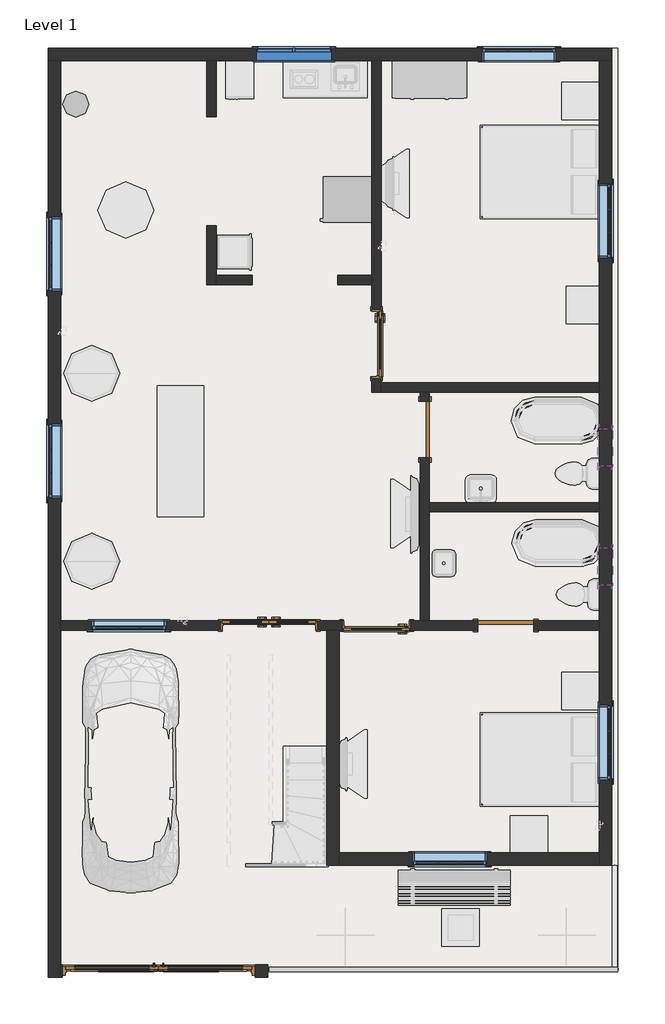
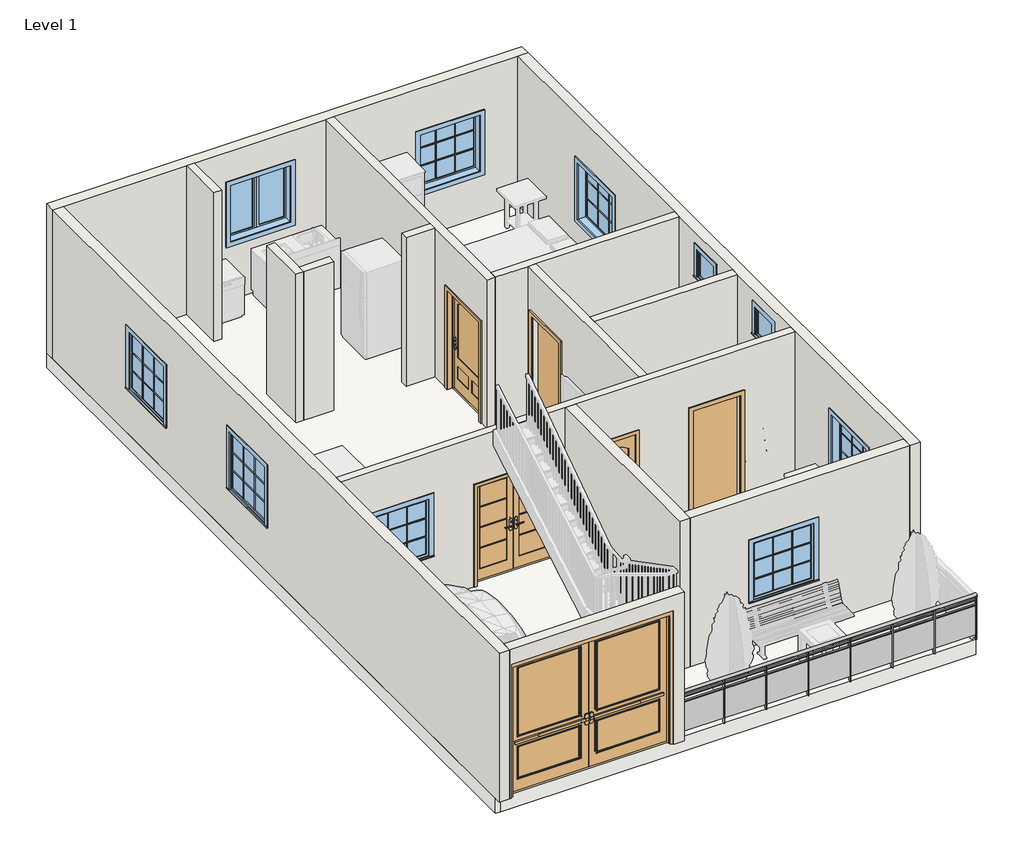
# One storey, part 1 of 3: 15 walls, 10 windows, 6 doors, 1 railing, 1 slab.
"""IFC4 building model written with IfcOpenShell, lengths in millimetres."""

from ifc_helpers import new_model, si_unit, point, frame, origin, origin_with_axes, place, context, project, spatial, polyline, ellipse_curve, trimmed, outline, extrude, faceted_brep, transform, mapped, element, save
from ifc_brep_helpers import plane_surface, extruded_surface, advanced_brep
from components import door_25c67de5, door_94998e6c, door_7b75190e, door_e43601eb, door_2971dfc0, door_686f89d2, window_7418cbd4, window_7e6ae3b0, window_0862ab64, window_e41d21a6

model = new_model("IFC4")

# Units and contexts
model_context = context("Model", 3, world=origin())
ifc_project = project(units=[si_unit("LENGTHUNIT", "METRE", prefix="MILLI")], contexts=[model_context])

# Site, building, storey
site = spatial("IfcSite", under=ifc_project)
building = spatial("IfcBuilding", under=site)
storey = spatial("IfcBuildingStorey", under=building, Name="Level 1", Elevation=0.0)

# Doors
placement = place(None, origin())
door_shape = door_25c67de5(model_context)
element("IfcDoor", 1, ObjectType="42\" x 80\"", at=placement, inside=storey, context=model_context, shape_type="MappedRepresentation", body=[
    mapped(door_shape, transform((-10170.509927, 3983.7437882, 0.0), x_axis=(1.0, 0.0, 0.0), y_axis=(0.0, 1.0, 0.0), z_axis=(0.0, 0.0, 1.0))),
])
element("IfcDoor", 2, ObjectType="42\" x 80\"", at=placement, inside=storey, context=model_context, shape_type="MappedRepresentation", body=[
    mapped(door_shape, transform((-10167.334927, 8584.3187882, 0.0), x_axis=(0.0, 1.0, 0.0), y_axis=(-1.0, 0.0, 0.0), z_axis=(0.0, 0.0, 1.0))),
])
door_2_shape = door_94998e6c(model_context)
element("IfcDoor", 3, ObjectType="Door-Exterior-Double-Full Glass-Wood_Clad : 60\" x 80\"", at=placement, inside=storey, context=model_context, shape_type="MappedRepresentation", body=[
    mapped(door_2_shape, transform((-11923.109927, 3990.0937882, 0.0), x_axis=(1.0, 0.0, 0.0), y_axis=(0.0, 1.0, 0.0), z_axis=(0.0, 0.0, 1.0))),
])
door_3_shape = door_7b75190e(model_context)
door_4_shape = door_e43601eb(model_context)
door_5_shape = door_2971dfc0(model_context)
element("IfcDoor", 4, ObjectType="Door-Exterior-Double-Two_Lite : 120\" x 104\"", at=placement, inside=storey, context=model_context, shape_type="MappedRepresentation", body=[
    mapped(door_3_shape, transform((-13726.509927, -1658.2312118, 0.0), x_axis=(1.0, 0.0, 0.0), y_axis=(0.0, 1.0, 0.0), z_axis=(0.0, 0.0, 1.0))),
    mapped(door_4_shape, transform((-13726.509927, -1658.2312118, 0.0), x_axis=(1.0, 0.0, 0.0), y_axis=(0.0, 1.0, 0.0), z_axis=(0.0, 0.0, 1.0))),
    mapped(door_5_shape, transform((-13726.509927, -1658.2312118, 0.0), x_axis=(1.0, 0.0, 0.0), y_axis=(0.0, 1.0, 0.0), z_axis=(0.0, 0.0, 1.0))),
])
door_6_shape = door_686f89d2(model_context)
element("IfcDoor", 5, ObjectType="Single-Flush : 36\" x 84\"", at=placement, inside=storey, context=model_context, shape_type="MappedRepresentation", body=[
    mapped(door_6_shape, transform((-9383.109927, 7187.3187882, 0.0), x_axis=(0.0, 1.0, 0.0), y_axis=(-1.0, 0.0, 0.0), z_axis=(0.0, 0.0, 1.0))),
])
element("IfcDoor", 6, ObjectType="Single-Flush : 36\" x 84\"", at=placement, inside=storey, context=model_context, shape_type="MappedRepresentation", body=[
    mapped(door_6_shape, transform((-8062.309927, 3986.9187882, 0.0), x_axis=(-1.0, 0.0, 0.0), y_axis=(0.0, -1.0, 0.0), z_axis=(0.0, 0.0, 1.0))),
])

# Railing
element("IfcRailing", 7, ObjectType="Glass Panel - Bottom Fill", at=placement, inside=storey, context=model_context, shape_type="SolidModel", body=[
    advanced_brep(
    [(-6233.509927, -1659.8187118, 914.4), (-6233.509927, -1583.6187118, 914.4), (-11923.109927, -1659.8187118, 914.4), (-11923.109927, -1583.6187118, 914.4)],
    [
        (0, 1, ellipse_curve(frame((-6233.509927, -1621.7187118, 914.4), z_axis=(1.0, 0.0, 0.0), x_axis=(0.0, 1.0, 0.0)), 38.1, 28.575)),
        (1, 0, ellipse_curve(frame((-6233.509927, -1621.7187118, 914.4), z_axis=(1.0, 0.0, 0.0), x_axis=(0.0, 1.0, 0.0)), 38.1, 28.575)),
        (2, 3, ellipse_curve(frame((-11923.109927, -1621.7187118, 914.4), z_axis=(-1.0, 0.0, 0.0), x_axis=(0.0, 1.0, 0.0)), 38.1, 28.575)),
        (3, 2, ellipse_curve(frame((-11923.109927, -1621.7187118, 914.4), z_axis=(-1.0, 0.0, 0.0), x_axis=(0.0, 1.0, 0.0)), 38.1, 28.575)),
        (0, 2),
        (3, 1),
    ],
    [
        plane_surface(frame((-6233.509927, -1621.7187118, 914.4), z_axis=(1.0, 0.0, 0.0), x_axis=(0.0, -1.0, 0.0))),
        plane_surface(frame((-11923.109927, -1621.7187118, 914.4), z_axis=(-1.0, 0.0, 0.0), x_axis=(0.0, -1.0, 0.0))),
        extruded_surface(trimmed(ellipse_curve(frame((-11923.109927, -1621.7187118, 914.4), z_axis=(1.0, 0.0, 0.0), x_axis=(0.0, 1.0, 0.0)), 38.1, 28.575), [point((-11923.109927, -1659.8187118, 914.4))], [point((-11923.109927, -1583.6187118, 914.4))], True, "CARTESIAN"), (5689.599999999999, 0.0, 0.0), 5689.599999999999),
        extruded_surface(trimmed(ellipse_curve(frame((-11923.109927, -1621.7187118, 914.4), z_axis=(1.0, 0.0, 0.0), x_axis=(0.0, 1.0, 0.0)), 38.1, 28.575), [point((-11923.109927, -1583.6187118, 914.4))], [point((-11923.109927, -1659.8187118, 914.4))], True, "CARTESIAN"), (5689.599999999999, 0.0, 0.0), 5689.599999999999),
    ],
    [
        (0, [[1, 2]]),
        (1, [[3, 4]]),
        (2, [[-1, 5, -4, 6]]),
        (3, [[-2, -6, -3, -5]]),
    ],
),
    extrude(outline(polyline([(-6233.509927, -1609.0187118), (-6233.509927, -1634.4187118), (-11923.109927, -1634.4187118), (-11923.109927, -1609.0187118), (-6233.509927, -1609.0187118)])), frame((0.0, 0.0, 800.1), z_axis=(0.0, 0.0, 1.0), x_axis=(1.0, 0.0, 0.0)), (0.0, 0.0, 1.0), 25.4),
    extrude(outline(polyline([(-6233.509927, -1609.0187118), (-6233.509927, -1634.4187118), (-11923.109927, -1634.4187118), (-11923.109927, -1609.0187118), (-6233.509927, -1609.0187118)])), frame((0.0, 0.0, 698.5), z_axis=(0.0, 0.0, 1.0), x_axis=(1.0, 0.0, 0.0)), (0.0, 0.0, 1.0), 25.4),
    extrude(outline(polyline([(-11110.309927, -1628.2538688), (-11923.109927, -1628.2538688), (-11923.109927, -1621.9038688), (-11110.309927, -1621.9038688), (-11110.309927, -1628.2538688)])), frame((0.0, 0.0, 101.6), z_axis=(0.0, 0.0, 1.0), x_axis=(1.0, 0.0, 0.0)), (0.0, 0.0, 1.0), 596.9),
    extrude(outline(polyline([(-11103.959927, -1596.3187118), (-11103.959927, -1647.1187118), (-11116.659927, -1647.1187118), (-11116.659927, -1596.3187118), (-11103.959927, -1596.3187118)])), origin_with_axes(), (0.0, 0.0, 1.0), 885.6788223),
    extrude(outline(polyline([(-10297.509927, -1628.2538688), (-11110.309927, -1628.2538688), (-11110.309927, -1621.9038688), (-10297.509927, -1621.9038688), (-10297.509927, -1628.2538688)])), frame((0.0, 0.0, 101.6), z_axis=(0.0, 0.0, 1.0), x_axis=(1.0, 0.0, 0.0)), (0.0, 0.0, 1.0), 596.9),
    extrude(outline(polyline([(-10291.159927, -1596.3187118), (-10291.159927, -1647.1187118), (-10303.859927, -1647.1187118), (-10303.859927, -1596.3187118), (-10291.159927, -1596.3187118)])), origin_with_axes(), (0.0, 0.0, 1.0), 885.6788223),
    extrude(outline(polyline([(-9484.709927, -1628.2538688), (-10297.509927, -1628.2538688), (-10297.509927, -1621.9038688), (-9484.709927, -1621.9038688), (-9484.709927, -1628.2538688)])), frame((0.0, 0.0, 101.6), z_axis=(0.0, 0.0, 1.0), x_axis=(1.0, 0.0, 0.0)), (0.0, 0.0, 1.0), 596.9),
    extrude(outline(polyline([(-9478.359927, -1596.3187118), (-9478.359927, -1647.1187118), (-9491.059927, -1647.1187118), (-9491.059927, -1596.3187118), (-9478.359927, -1596.3187118)])), origin_with_axes(), (0.0, 0.0, 1.0), 885.6788223),
    extrude(outline(polyline([(-8671.909927, -1628.2538688), (-9484.709927, -1628.2538688), (-9484.709927, -1621.9038688), (-8671.909927, -1621.9038688), (-8671.909927, -1628.2538688)])), frame((0.0, 0.0, 101.6), z_axis=(0.0, 0.0, 1.0), x_axis=(1.0, 0.0, 0.0)), (0.0, 0.0, 1.0), 596.9),
    extrude(outline(polyline([(-8665.559927, -1596.3187118), (-8665.559927, -1647.1187118), (-8678.259927, -1647.1187118), (-8678.259927, -1596.3187118), (-8665.559927, -1596.3187118)])), origin_with_axes(), (0.0, 0.0, 1.0), 885.6788223),
    extrude(outline(polyline([(-7859.109927, -1628.2538688), (-8671.909927, -1628.2538688), (-8671.909927, -1621.9038688), (-7859.109927, -1621.9038688), (-7859.109927, -1628.2538688)])), frame((0.0, 0.0, 101.6), z_axis=(0.0, 0.0, 1.0), x_axis=(1.0, 0.0, 0.0)), (0.0, 0.0, 1.0), 596.9),
    extrude(outline(polyline([(-7852.759927, -1596.3187118), (-7852.759927, -1647.1187118), (-7865.459927, -1647.1187118), (-7865.459927, -1596.3187118), (-7852.759927, -1596.3187118)])), origin_with_axes(), (0.0, 0.0, 1.0), 885.6788223),
    extrude(outline(polyline([(-7046.309927, -1628.2538688), (-7859.109927, -1628.2538688), (-7859.109927, -1621.9038688), (-7046.309927, -1621.9038688), (-7046.309927, -1628.2538688)])), frame((0.0, 0.0, 101.6), z_axis=(0.0, 0.0, 1.0), x_axis=(1.0, 0.0, 0.0)), (0.0, 0.0, 1.0), 596.9),
    extrude(outline(polyline([(-7039.959927, -1596.3187118), (-7039.959927, -1647.1187118), (-7052.659927, -1647.1187118), (-7052.659927, -1596.3187118), (-7039.959927, -1596.3187118)])), origin_with_axes(), (0.0, 0.0, 1.0), 885.6788223),
    extrude(outline(polyline([(-6233.509927, -1628.2538688), (-7046.309927, -1628.2538688), (-7046.309927, -1621.9038688), (-6233.509927, -1621.9038688), (-6233.509927, -1628.2538688)])), frame((0.0, 0.0, 101.6), z_axis=(0.0, 0.0, 1.0), x_axis=(1.0, 0.0, 0.0)), (0.0, 0.0, 1.0), 596.9),
    extrude(outline(polyline([(-11910.409927, -1612.1937118), (-11910.409927, -1631.2437118), (-11929.459927, -1631.2437118), (-11929.459927, -1612.1937118), (-11910.409927, -1612.1937118)])), origin_with_axes(), (0.0, 0.0, 1.0), 885.6788223),
    extrude(outline(polyline([(-6227.159927, -1612.1937118), (-6227.159927, -1631.2437118), (-6246.209927, -1631.2437118), (-6246.209927, -1612.1937118), (-6227.159927, -1612.1937118)])), origin_with_axes(), (0.0, 0.0, 1.0), 885.6788223),
])

# Slab
element("IfcSlab", 8, ObjectType="Generic - 12\"", at=placement, inside=storey, context=model_context, shape_type="SweptSolid", body=[
    extrude(outline(polyline([(-6233.509927, 13410.3187882), (-6233.509927, -1621.7187118), (-15428.309927, -1621.7187118), (-15529.909927, -1621.7187118), (-15529.909927, 13410.3187882), (-6233.509927, 13410.3187882)])), frame((0.0, 0.0, -304.8), z_axis=(0.0, 0.0, 1.0), x_axis=(1.0, 0.0, 0.0)), (0.0, 0.0, 1.0), 304.8),
])

# Walls
element("IfcWall", 9, ObjectType="Generic - 8\"", at=placement, inside=storey, context=model_context, shape_type="Brep", body=[
    faceted_brep([(-15529.909927, 13207.1187882, 0.0), (-15326.709927, 13207.1187882, 0.0), (-12939.109927, 13207.1187882, 0.0), (-12786.709927, 13207.1187882, 0.0), (-10246.709927, 13207.1187882, 0.0), (-10094.309927, 13207.1187882, 0.0), (-6538.309927, 13207.1187882, 0.0), (-6335.109927, 13207.1187882, 0.0), (-6335.109927, 13207.1187882, 3048.0), (-6538.309927, 13207.1187882, 3048.0), (-10094.309927, 13207.1187882, 3048.0), (-10246.709927, 13207.1187882, 3048.0), (-12786.709927, 13207.1187882, 3048.0), (-12939.109927, 13207.1187882, 3048.0), (-15326.709927, 13207.1187882, 3048.0), (-15529.909927, 13207.1187882, 3048.0), (-7236.809927, 13207.1187882, 2133.6), (-7236.809927, 13207.1187882, 914.4), (-8456.009927, 13207.1187882, 914.4), (-8456.009927, 13207.1187882, 2133.6), (-10907.109927, 13207.1187882, 2387.6), (-10907.109927, 13207.1187882, 1168.4), (-12126.309927, 13207.1187882, 1168.4), (-12126.309927, 13207.1187882, 2387.6), (-15529.909927, 13410.3187882, 0.0), (-15529.909927, 13410.3187882, 3048.0), (-6335.109927, 13410.3187882, 3048.0), (-6335.109927, 13410.3187882, 0.0), (-7236.809927, 13410.3187882, 2133.6), (-8456.009927, 13410.3187882, 2133.6), (-8456.009927, 13410.3187882, 914.4), (-7236.809927, 13410.3187882, 914.4), (-10907.109927, 13410.3187882, 2387.6), (-12126.309927, 13410.3187882, 2387.6), (-12126.309927, 13410.3187882, 1168.4), (-10907.109927, 13410.3187882, 1168.4)], [[[0, 1, 2, 3, 4, 5, 6, 7, 8, 9, 10, 11, 12, 13, 14, 15], [16, 17, 18, 19], [20, 21, 22, 23]], [[24, 25, 26, 27], [28, 29, 30, 31], [32, 33, 34, 35]], [[7, 6, 5, 4, 3, 2, 1, 0, 24, 27]], [[15, 14, 13, 12, 11, 10, 9, 8, 26, 25]], [[8, 7, 27, 26]], [[0, 15, 25, 24]], [[17, 16, 28, 31]], [[18, 17, 31, 30]], [[19, 18, 30, 29]], [[16, 19, 29, 28]], [[21, 20, 32, 35]], [[22, 21, 35, 34]], [[23, 22, 34, 33]], [[20, 23, 33, 32]]]),
])
element("IfcWall", 10, ObjectType="Generic - 8\"", at=placement, inside=storey, context=model_context, shape_type="Brep", body=[
    faceted_brep([(-6538.309927, 13207.1187882, 0.0), (-6538.309927, 7949.3187882, 0.0), (-6538.309927, 7796.9187882, 0.0), (-6538.309927, 5993.5187882, 0.0), (-6538.309927, 5841.1187882, 0.0), (-6538.309927, 4063.1187882, 0.0), (-6538.309927, 3910.7187882, 0.0), (-6538.309927, 278.5187882, 0.0), (-6538.309927, 75.3187882, 0.0), (-6538.309927, 75.3187882, 3048.0), (-6538.309927, 278.5187882, 3048.0), (-6538.309927, 3910.7187882, 3048.0), (-6538.309927, 4063.1187882, 3048.0), (-6538.309927, 5841.1187882, 3048.0), (-6538.309927, 5993.5187882, 3048.0), (-6538.309927, 7796.9187882, 3048.0), (-6538.309927, 7949.3187882, 3048.0), (-6538.309927, 13207.1187882, 3048.0), (-6538.309927, 1472.3187882, 2133.6), (-6538.309927, 1472.3187882, 914.4), (-6538.309927, 2691.5187882, 914.4), (-6538.309927, 2691.5187882, 2133.6), (-6538.309927, 9981.3187882, 2133.6), (-6538.309927, 9981.3187882, 914.4), (-6538.309927, 11200.5187882, 914.4), (-6538.309927, 11200.5187882, 2133.6), (-6538.309927, 7200.0187882, 2768.6), (-6538.309927, 6590.4187882, 2768.6), (-6538.309927, 6590.4187882, 2159.0), (-6538.309927, 7200.0187882, 2159.0), (-6538.309927, 5256.9187882, 2768.6), (-6538.309927, 4647.3187882, 2768.6), (-6538.309927, 4647.3187882, 2159.0), (-6538.309927, 5256.9187882, 2159.0), (-6335.109927, 13207.1187882, 0.0), (-6335.109927, 13207.1187882, 3048.0), (-6335.109927, 75.3187882, 3048.0), (-6335.109927, 75.3187882, 0.0), (-6335.109927, 1472.3187882, 2133.6), (-6335.109927, 2691.5187882, 2133.6), (-6335.109927, 2691.5187882, 914.4), (-6335.109927, 1472.3187882, 914.4), (-6335.109927, 9981.3187882, 2133.6), (-6335.109927, 11200.5187882, 2133.6), (-6335.109927, 11200.5187882, 914.4), (-6335.109927, 9981.3187882, 914.4), (-6335.109927, 7200.0187882, 2768.6), (-6335.109927, 7200.0187882, 2159.0), (-6335.109927, 6590.4187882, 2159.0), (-6335.109927, 6590.4187882, 2768.6), (-6335.109927, 5256.9187882, 2768.6), (-6335.109927, 5256.9187882, 2159.0), (-6335.109927, 4647.3187882, 2159.0), (-6335.109927, 4647.3187882, 2768.6)], [[[0, 1, 2, 3, 4, 5, 6, 7, 8, 9, 10, 11, 12, 13, 14, 15, 16, 17], [18, 19, 20, 21], [22, 23, 24, 25], [26, 27, 28, 29], [30, 31, 32, 33]], [[34, 35, 36, 37], [38, 39, 40, 41], [42, 43, 44, 45], [46, 47, 48, 49], [50, 51, 52, 53]], [[8, 7, 6, 5, 4, 3, 2, 1, 0, 34, 37]], [[17, 16, 15, 14, 13, 12, 11, 10, 9, 36, 35]], [[0, 17, 35, 34]], [[9, 8, 37, 36]], [[19, 18, 38, 41]], [[20, 19, 41, 40]], [[21, 20, 40, 39]], [[18, 21, 39, 38]], [[23, 22, 42, 45]], [[24, 23, 45, 44]], [[25, 24, 44, 43]], [[22, 25, 43, 42]], [[47, 46, 26, 29]], [[48, 47, 29, 28]], [[49, 48, 28, 27]], [[46, 49, 27, 26]], [[51, 50, 30, 33]], [[52, 51, 33, 32]], [[53, 52, 32, 31]], [[50, 53, 31, 30]]]),
])
element("IfcWall", 11, ObjectType="Generic - 8\"", at=placement, inside=storey, context=model_context, shape_type="SweptSolid", body=[
    extrude(outline(polyline([(0.0, -6538.309927), (3048.0, -6538.309927), (3048.0, -10780.109927), (0.0, -10780.109927), (0.0, -6538.309927)]), holes=[polyline([(2133.6, -9586.309927), (2133.6, -8367.109927), (914.4, -8367.109927), (914.4, -9586.309927), (2133.6, -9586.309927)])]), frame((0.0, 75.3187882, 0.0), z_axis=(0.0, 1.0, 0.0), x_axis=(0.0, 0.0, 1.0)), (0.0, 0.0, 1.0), 203.2),
])
element("IfcWall", 12, ObjectType="Generic - 8\"", at=placement, inside=storey, context=model_context, shape_type="Brep", body=[
    faceted_brep([(-15326.709927, -1753.4812118, 0.0), (-15326.709927, -1550.2812118, 0.0), (-15326.709927, 3910.7187882, 0.0), (-15326.709927, 4063.1187882, 0.0), (-15326.709927, 13207.1187882, 0.0), (-15326.709927, 13207.1187882, 3048.0), (-15326.709927, 4063.1187882, 3048.0), (-15326.709927, 3910.7187882, 3048.0), (-15326.709927, -1550.2812118, 3048.0), (-15326.709927, -1753.4812118, 3048.0), (-15326.709927, 7282.5687882, 2133.6), (-15326.709927, 7282.5687882, 914.4), (-15326.709927, 6063.3687882, 914.4), (-15326.709927, 6063.3687882, 2133.6), (-15326.709927, 10660.7687882, 2133.6), (-15326.709927, 10660.7687882, 914.4), (-15326.709927, 9441.5687882, 914.4), (-15326.709927, 9441.5687882, 2133.6), (-15529.909927, -1753.4812118, 0.0), (-15529.909927, -1753.4812118, 3048.0), (-15529.909927, 13207.1187882, 3048.0), (-15529.909927, 13207.1187882, 0.0), (-15529.909927, 7282.5687882, 2133.6), (-15529.909927, 6063.3687882, 2133.6), (-15529.909927, 6063.3687882, 914.4), (-15529.909927, 7282.5687882, 914.4), (-15529.909927, 10660.7687882, 2133.6), (-15529.909927, 9441.5687882, 2133.6), (-15529.909927, 9441.5687882, 914.4), (-15529.909927, 10660.7687882, 914.4)], [[[0, 1, 2, 3, 4, 5, 6, 7, 8, 9], [10, 11, 12, 13], [14, 15, 16, 17]], [[18, 19, 20, 21], [22, 23, 24, 25], [26, 27, 28, 29]], [[4, 3, 2, 1, 0, 18, 21]], [[9, 8, 7, 6, 5, 20, 19]], [[5, 4, 21, 20]], [[11, 10, 22, 25]], [[12, 11, 25, 24]], [[13, 12, 24, 23]], [[10, 13, 23, 22]], [[15, 14, 26, 29]], [[16, 15, 29, 28]], [[17, 16, 28, 27]], [[14, 17, 27, 26]], [[0, 9, 19, 18]]]),
])
element("IfcWall", 13, ObjectType="Generic - 8\"", at=placement, inside=storey, context=model_context, shape_type="Brep", body=[
    faceted_brep([(-10983.309927, 3910.7187882, 0.0), (-10983.309927, 75.3187882, 0.0), (-10983.309927, 75.3187882, 3048.0), (-10983.309927, 3910.7187882, 3048.0), (-10780.109927, 3910.7187882, 0.0), (-10780.109927, 3910.7187882, 3048.0), (-10780.109927, 278.5187882, 3048.0), (-10780.109927, 75.3187882, 3048.0), (-10780.109927, 75.3187882, 0.0), (-10780.109927, 278.5187882, 0.0)], [[[0, 1, 2, 3]], [[4, 5, 6, 7, 8, 9]], [[1, 0, 4, 9, 8]], [[3, 2, 7, 6, 5]], [[0, 3, 5, 4]], [[2, 1, 8, 7]]]),
])
element("IfcWall", 14, ObjectType="Generic - 8\"", at=placement, inside=storey, context=model_context, shape_type="SweptSolid", body=[
    extrude(outline(polyline([(0.0, -11948.509927), (3048.0, -11948.509927), (3048.0, -15326.709927), (0.0, -15326.709927), (0.0, -15301.309927), (2743.2, -15301.309927), (2743.2, -12151.709927), (0.0, -12151.709927), (0.0, -11948.509927)])), frame((0.0, -1753.4812118, 0.0), z_axis=(0.0, 1.0, 0.0), x_axis=(0.0, 0.0, 1.0)), (0.0, 0.0, 1.0), 203.2),
])
element("IfcWall", 15, ObjectType="INNER WALL", at=placement, inside=storey, context=model_context, shape_type="Brep", body=[
    faceted_brep([(-10246.709927, 7796.9187882, 3048.0), (-10246.709927, 9549.5187882, 3048.0), (-10246.709927, 9701.9187882, 3048.0), (-10246.709927, 13207.1187882, 3048.0), (-10246.709927, 13207.1187882, 0.0), (-10246.709927, 9701.9187882, 0.0), (-10246.709927, 9549.5187882, 0.0), (-10246.709927, 9143.1187882, 0.0), (-10246.709927, 9143.1187882, 2057.4), (-10246.709927, 8025.5187882, 2057.4), (-10246.709927, 8025.5187882, 0.0), (-10246.709927, 7796.9187882, 0.0), (-10094.309927, 13207.1187882, 3048.0), (-10094.309927, 7949.3187882, 3048.0), (-10094.309927, 7796.9187882, 3048.0), (-10094.309927, 7796.9187882, 0.0), (-10094.309927, 7949.3187882, 0.0), (-10094.309927, 8025.5187882, 0.0), (-10094.309927, 8025.5187882, 2057.4), (-10094.309927, 9143.1187882, 2057.4), (-10094.309927, 9143.1187882, 0.0), (-10094.309927, 13207.1187882, 0.0)], [[[0, 1, 2, 3, 4, 5, 6, 7, 8, 9, 10, 11]], [[12, 13, 14, 15, 16, 17, 18, 19, 20, 21]], [[4, 21, 20, 7, 6, 5]], [[15, 11, 10, 17, 16]], [[3, 2, 1, 0, 14, 13, 12]], [[4, 3, 12, 21]], [[0, 11, 15, 14]], [[19, 8, 7, 20]], [[8, 19, 18, 9]], [[9, 18, 17, 10]]]),
])
element("IfcWall", 16, ObjectType="INNER WALL", at=placement, inside=storey, context=model_context, shape_type="Brep", body=[
    faceted_brep([(-10094.309927, 7796.9187882, 0.0), (-9459.309927, 7796.9187882, 0.0), (-9306.909927, 7796.9187882, 0.0), (-6538.309927, 7796.9187882, 0.0), (-6538.309927, 7796.9187882, 3048.0), (-9306.909927, 7796.9187882, 3048.0), (-9459.309927, 7796.9187882, 3048.0), (-10094.309927, 7796.9187882, 3048.0), (-10094.309927, 7949.3187882, 0.0), (-10094.309927, 7949.3187882, 3048.0), (-6538.309927, 7949.3187882, 3048.0), (-6538.309927, 7949.3187882, 0.0)], [[[0, 1, 2, 3, 4, 5, 6, 7]], [[8, 9, 10, 11]], [[3, 2, 1, 0, 8, 11]], [[7, 6, 5, 4, 10, 9]], [[0, 7, 9, 8]], [[4, 3, 11, 10]]]),
])
element("IfcWall", 17, ObjectType="INNER WALL", at=placement, inside=storey, context=model_context, shape_type="Brep", body=[
    faceted_brep([(-15326.709927, 4063.1187882, 3048.0), (-9459.309927, 4063.1187882, 3048.0), (-9306.909927, 4063.1187882, 3048.0), (-6538.309927, 4063.1187882, 3048.0), (-6538.309927, 4063.1187882, 0.0), (-7605.109927, 4063.1187882, 0.0), (-7605.109927, 4063.1187882, 2133.6), (-8519.509927, 4063.1187882, 2133.6), (-8519.509927, 4063.1187882, 0.0), (-9306.909927, 4063.1187882, 0.0), (-9459.309927, 4063.1187882, 0.0), (-9611.709927, 4063.1187882, 0.0), (-9611.709927, 4063.1187882, 2057.4), (-10729.309927, 4063.1187882, 2057.4), (-10729.309927, 4063.1187882, 0.0), (-11135.709927, 4063.1187882, 0.0), (-11135.709927, 4063.1187882, 2057.4), (-12710.509927, 4063.1187882, 2057.4), (-12710.509927, 4063.1187882, 0.0), (-15326.709927, 4063.1187882, 0.0), (-14818.709927, 4063.1187882, 2133.6), (-14818.709927, 4063.1187882, 914.4), (-13599.509927, 4063.1187882, 914.4), (-13599.509927, 4063.1187882, 2133.6), (-6538.309927, 3910.7187882, 3048.0), (-10780.109927, 3910.7187882, 3048.0), (-10983.309927, 3910.7187882, 3048.0), (-15326.709927, 3910.7187882, 3048.0), (-15326.709927, 3910.7187882, 0.0), (-12710.509927, 3910.7187882, 0.0), (-12710.509927, 3910.7187882, 2057.4), (-11135.709927, 3910.7187882, 2057.4), (-11135.709927, 3910.7187882, 0.0), (-10983.309927, 3910.7187882, 0.0), (-10780.109927, 3910.7187882, 0.0), (-10729.309927, 3910.7187882, 0.0), (-10729.309927, 3910.7187882, 2057.4), (-9611.709927, 3910.7187882, 2057.4), (-9611.709927, 3910.7187882, 0.0), (-8519.509927, 3910.7187882, 0.0), (-8519.509927, 3910.7187882, 2133.6), (-7605.109927, 3910.7187882, 2133.6), (-7605.109927, 3910.7187882, 0.0), (-6538.309927, 3910.7187882, 0.0), (-14818.709927, 3910.7187882, 2133.6), (-13599.509927, 3910.7187882, 2133.6), (-13599.509927, 3910.7187882, 914.4), (-14818.709927, 3910.7187882, 914.4)], [[[0, 1, 2, 3, 4, 5, 6, 7, 8, 9, 10, 11, 12, 13, 14, 15, 16, 17, 18, 19], [20, 21, 22, 23]], [[24, 25, 26, 27, 28, 29, 30, 31, 32, 33, 34, 35, 36, 37, 38, 39, 40, 41, 42, 43], [44, 45, 46, 47]], [[4, 43, 42, 5]], [[28, 19, 18, 29]], [[8, 39, 38, 11, 10, 9]], [[14, 35, 34, 33, 32, 15]], [[3, 2, 1, 0, 27, 26, 25, 24]], [[4, 3, 24, 43]], [[0, 19, 28, 27]], [[40, 39, 8, 7]], [[41, 40, 7, 6]], [[42, 41, 6, 5]], [[37, 12, 11, 38]], [[12, 37, 36, 13]], [[13, 36, 35, 14]], [[21, 20, 44, 47]], [[22, 21, 47, 46]], [[23, 22, 46, 45]], [[20, 23, 45, 44]], [[31, 16, 15, 32]], [[16, 31, 30, 17]], [[17, 30, 29, 18]]]),
])
element("IfcWall", 18, ObjectType="INNER WALL", at=placement, inside=storey, context=model_context, shape_type="Brep", body=[
    faceted_brep([(-9459.309927, 7796.9187882, 0.0), (-9459.309927, 7644.5187882, 0.0), (-9459.309927, 7644.5187882, 2133.6), (-9459.309927, 6730.1187882, 2133.6), (-9459.309927, 6730.1187882, 0.0), (-9459.309927, 4063.1187882, 0.0), (-9459.309927, 4063.1187882, 3048.0), (-9459.309927, 7796.9187882, 3048.0), (-9306.909927, 7644.5187882, 2133.6), (-9306.909927, 7644.5187882, 0.0), (-9306.909927, 7796.9187882, 0.0), (-9306.909927, 7796.9187882, 3048.0), (-9306.909927, 5993.5187882, 3048.0), (-9306.909927, 5841.1187882, 3048.0), (-9306.909927, 4063.1187882, 3048.0), (-9306.909927, 4063.1187882, 0.0), (-9306.909927, 5841.1187882, 0.0), (-9306.909927, 5993.5187882, 0.0), (-9306.909927, 6730.1187882, 0.0), (-9306.909927, 6730.1187882, 2133.6)], [[[0, 1, 2, 3, 4, 5, 6, 7]], [[8, 9, 10, 11, 12, 13, 14, 15, 16, 17, 18, 19]], [[10, 9, 1, 0]], [[18, 17, 16, 15, 5, 4]], [[7, 6, 14, 13, 12, 11]], [[0, 7, 11, 10]], [[6, 5, 15, 14]], [[2, 1, 9, 8]], [[3, 2, 8, 19]], [[4, 3, 19, 18]]]),
])
element("IfcWall", 19, ObjectType="INNER WALL", at=placement, inside=storey, context=model_context, shape_type="SweptSolid", body=[
    extrude(outline(polyline([(-6538.309927, 5841.1187882), (-9306.909927, 5841.1187882), (-9306.909927, 5993.5187882), (-6538.309927, 5993.5187882), (-6538.309927, 5841.1187882)])), origin_with_axes(), (0.0, 0.0, 1.0), 3048.0),
])
element("IfcWall", 20, ObjectType="INNER WALL", at=placement, inside=storey, context=model_context, shape_type="SweptSolid", body=[
    extrude(outline(polyline([(-12939.109927, 12292.7187882), (-12939.109927, 13207.1187882), (-12786.709927, 13207.1187882), (-12786.709927, 12292.7187882), (-12939.109927, 12292.7187882)])), origin_with_axes(), (0.0, 0.0, 1.0), 3048.0),
])
element("IfcWall", 21, ObjectType="INNER WALL", at=placement, inside=storey, context=model_context, shape_type="SweptSolid", body=[
    extrude(outline(polyline([(-12202.509927, 9549.5187882), (-12786.709927, 9549.5187882), (-12786.709927, 9701.9187882), (-12202.509927, 9701.9187882), (-12202.509927, 9549.5187882)])), origin_with_axes(), (0.0, 0.0, 1.0), 3048.0),
])
element("IfcWall", 22, ObjectType="INNER WALL", at=placement, inside=storey, context=model_context, shape_type="SweptSolid", body=[
    extrude(outline(polyline([(-10246.709927, 9549.5187882), (-10805.509927, 9549.5187882), (-10805.509927, 9701.9187882), (-10246.709927, 9701.9187882), (-10246.709927, 9549.5187882)])), origin_with_axes(), (0.0, 0.0, 1.0), 3048.0),
])
element("IfcWall", 23, ObjectType="INNER WALL", at=placement, inside=storey, context=model_context, shape_type="Brep", body=[
    faceted_brep([(-12939.109927, 10514.7187882, 0.0), (-12939.109927, 9549.5187882, 0.0), (-12939.109927, 9549.5187882, 3048.0), (-12939.109927, 10514.7187882, 3048.0), (-12786.709927, 10514.7187882, 0.0), (-12786.709927, 10514.7187882, 3048.0), (-12786.709927, 9701.9187882, 3048.0), (-12786.709927, 9549.5187882, 3048.0), (-12786.709927, 9549.5187882, 0.0), (-12786.709927, 9701.9187882, 0.0)], [[[0, 1, 2, 3]], [[4, 5, 6, 7, 8, 9]], [[1, 0, 4, 9, 8]], [[3, 2, 7, 6, 5]], [[0, 3, 5, 4]], [[2, 1, 8, 7]]]),
])

# Windows
window_shape = window_7418cbd4(model_context)
element("IfcWindow", 24, ObjectType="Casement 3x3 with Trim : 48\" x 48\"", at=placement, inside=storey, context=model_context, shape_type="MappedRepresentation", body=[
    mapped(window_shape, transform((-8976.709927, 176.9187882, 0.0), x_axis=(-1.0, 0.0, 0.0), y_axis=(0.0, -1.0, 0.0), z_axis=(0.0, 0.0, 1.0))),
])
element("IfcWindow", 25, ObjectType="Casement 3x3 with Trim : 48\" x 48\"", at=placement, inside=storey, context=model_context, shape_type="MappedRepresentation", body=[
    mapped(window_shape, transform((-6436.709927, 2081.9187882, 0.0), x_axis=(0.0, -1.0, 0.0), y_axis=(1.0, 0.0, 0.0), z_axis=(0.0, 0.0, 1.0))),
])
element("IfcWindow", 26, ObjectType="Casement 3x3 with Trim : 48\" x 48\"", at=placement, inside=storey, context=model_context, shape_type="MappedRepresentation", body=[
    mapped(window_shape, transform((-6436.709927, 10590.9187882, 0.0), x_axis=(0.0, -1.0, 0.0), y_axis=(1.0, 0.0, 0.0), z_axis=(0.0, 0.0, 1.0))),
])
element("IfcWindow", 27, ObjectType="Casement 3x3 with Trim : 48\" x 48\"", at=placement, inside=storey, context=model_context, shape_type="MappedRepresentation", body=[
    mapped(window_shape, transform((-7846.409927, 13308.7187882, 0.0), x_axis=(1.0, 0.0, 0.0), y_axis=(0.0, 1.0, 0.0), z_axis=(0.0, 0.0, 1.0))),
])
element("IfcWindow", 28, ObjectType="Casement 3x3 with Trim : 48\" x 48\"", at=placement, inside=storey, context=model_context, shape_type="MappedRepresentation", body=[
    mapped(window_shape, transform((-15428.309927, 6672.9687882, 0.0), x_axis=(0.0, 1.0, 0.0), y_axis=(-1.0, 0.0, 0.0), z_axis=(0.0, 0.0, 1.0))),
])
element("IfcWindow", 29, ObjectType="Casement 3x3 with Trim : 48\" x 48\"", at=placement, inside=storey, context=model_context, shape_type="MappedRepresentation", body=[
    mapped(window_shape, transform((-15428.309927, 10051.1687882, 0.0), x_axis=(0.0, 1.0, 0.0), y_axis=(-1.0, 0.0, 0.0), z_axis=(0.0, 0.0, 1.0))),
])
window_2_shape = window_7e6ae3b0(model_context)
element("IfcWindow", 30, ObjectType="Casement 3x3 with Trim : 48\" x 48\"", at=placement, inside=storey, context=model_context, shape_type="MappedRepresentation", body=[
    mapped(window_2_shape, transform((-14209.109927, 3986.9187882, 0.0), x_axis=(-1.0, 0.0, 0.0), y_axis=(0.0, -1.0, 0.0), z_axis=(0.0, 0.0, 1.0))),
])
window_3_shape = window_0862ab64(model_context)
element("IfcWindow", 31, ObjectType="Casement Dbl with Trim : 48\" x 48\"", at=placement, inside=storey, context=model_context, shape_type="MappedRepresentation", body=[
    mapped(window_3_shape, transform((-11516.709927, 13289.6687882, 254.0), x_axis=(1.0, 0.0, 0.0), y_axis=(0.0, 1.0, 0.0), z_axis=(0.0, 0.0, 1.0))),
])
window_4_shape = window_e41d21a6(model_context)
element("IfcWindow", 32, ObjectType="Transom with Trim : 24\" x 24\"", at=placement, inside=storey, context=model_context, shape_type="MappedRepresentation", body=[
    mapped(window_4_shape, transform((-6436.709927, 6933.3187882, 0.0), x_axis=(0.0, 1.0, 0.0), y_axis=(-1.0, 0.0, 0.0), z_axis=(0.0, 0.0, 1.0))),
])
element("IfcWindow", 33, ObjectType="Transom with Trim : 24\" x 24\"", at=placement, inside=storey, context=model_context, shape_type="MappedRepresentation", body=[
    mapped(window_4_shape, transform((-6436.709927, 4990.2187882, 0.0), x_axis=(0.0, 1.0, 0.0), y_axis=(-1.0, 0.0, 0.0), z_axis=(0.0, 0.0, 1.0))),
])

save(model, "model.ifc")

# Revit data of these elements
# Type "42\" x 80\""
#   Type Mark = "8"
#   Assembly Code = "B2030100"
#   Analytic Construction = "French door, wood frame with single glass"
#   Threshold Offset [instance default] = 0' - 0 1/2"
#   Thickness = 0' - 1 3/8"
#   Thermal Resistance (R) = 1.0696 (h·ft²·°F)/BTU
#   Swing Angle [instance default] = 90.00°
#   Stiles = 0' - 4 3/4"
#   Rough Width = 3' - 8"
#   Rough Height = 6' - 9"
#   Radius = 2' - 4 29/32"
#   Lock Rail = 0' - 7 1/8"
#   Height = 6' - 8"
#   Width = 3' - 6"
#   Heat Transfer Coefficient (U) = 0.9350 BTU/(h·ft²·°F)
#   Door Offset [instance default] = 0' - 0"
#   Bottom Rail = 0' - 9 1/2"
#   Threshold [instance default] = yes
#   Function = 1
#   Exterior Trim [instance default] = yes
#   Trim Material = Cherry
#   Threshold Material = Cherry
#   Panel Material = Cherry
#   Glazing = Glass
#   Frame Material = Cherry
#   Door Handle Material = Aluminum
#   Visual Light Transmittance = 0
#   Solar Heat Gain Coefficient = 0
#   Wall Closure = (empty or 0)
#   Construction Type = (empty or 0)
# Type "Door-Exterior-Double-Full Glass-Wood_Clad : 60\" x 80\""
#   Type Mark = "9"
#   Assembly Code = "B2030100"
#   Analytic Construction = "French door, wood frame with double glass"
#   Top Rail = 0' - 4 11/16"
#   Threshold Offset [instance default] = 0' - 0 1/2"
#   Thickness = 0' - 1 3/8"
#   Thermal Resistance (R) = 1.9158 (h·ft²·°F)/BTU
#   Swing Angle [instance default] = 90.00°
#   Stiles = 0' - 4 3/4"
#   Rough Width = 5' - 2"
#   Rough Height = 6' - 9"
#   Panel Width = 2' - 6"
#   Door Offset [instance default] = 0' - 0"
#   Height = 6' - 8"
#   Width = 5' - 0"
#   Heat Transfer Coefficient (U) = 0.5220 BTU/(h·ft²·°F)
#   Bottom Rail = 0' - 9 1/8"
#   Exterior Trim [instance default] = yes
#   Threshold [instance default] = yes
#   Show Grill [instance default] = yes
#   Function = 1
#   Trim Material = Cherry
#   Threshold Material = Cherry
#   Panel Material = Cherry
#   Glazing = Glass
#   Frame Material = Cherry
#   Door Handle Material = Aluminum
#   Visual Light Transmittance = 0
#   Solar Heat Gain Coefficient = 0
#   Wall Closure = (empty or 0)
#   Construction Type = (empty or 0)
# Type "Door-Exterior-Double-Two_Lite : 120\" x 104\""
#   Type Mark = "10"
#   Assembly Code = "B2030100"
#   Analytic Construction = "Metal frame, double glass door"
#   Top Rail = 0' - 4 5/8"
#   Threshold Length [instance default] = 10' - 4"
#   Threshold Offset [instance default] = 0' - 0 1/2"
#   Thickness = 0' - 1 3/4"
#   Thermal Resistance (R) = 1.3794 (h·ft²·°F)/BTU
#   Swing Angle [instance default] = 90.00°
#   Strike Height = 3' - 4"
#   Stiles = 0' - 6"
#   SinglePanelWidth = 5' - 0"
#   Rough Width [instance default] = 10' - 4"
#   Rough Height [instance default] = 9' - 0"
#   MFOpeningHeight [instance default] = 0' - 4"
#   MFOpeningWidth [instance default] = 0' - 4"
#   Lock Rail = 0' - 8"
#   Inset Calculate [instance default] = 0' - 4"
#   Masonry Inset [instance default] = 0' - 1"
#   Height = 8' - 8"
#   Width = 10' - 0"
#   Heat Transfer Coefficient (U) = 0.7250 BTU/(h·ft²·°F)
#   Glass Thickness = 0' - 0 3/4"
#   Masonry Frame Depth = 0' - 5 3/4"
#   Bottom Rail = 0' - 10"
#   Threshold [instance default] = yes
#   Masonry Frame [instance default] = yes
#   Function = 1
#   Dry Wall Frame [instance default] = no
#   Threshold Material = none
#   Panic Bar Material = Metal - Stainless Steel
#   Panel Material = Metal - Painted - Grey
#   Glass Stop Material = Metal - Painted - Grey
#   Frame Material = Metal - Painted - Grey
#   Exterior Pull Material = Metal - Stainless Steel
#   Visual Light Transmittance = 0
#   Solar Heat Gain Coefficient = 0
#   Wall Closure = (empty or 0)
# Type "Single-Flush : 36\" x 84\""
#   Type Mark = "1"
#   Construction Type Id = "MDOOR"
#   Assembly Code = "C1020"
#   Analytic Construction = "Metal"
#   Thickness = 0' - 2"
#   Heat Transfer Coefficient (U) = 0.651978 BTU/(h·ft²·°F)
#   Height = 7' - 0"
#   Trim Projection Ext = 0' - 1"
#   Trim Projection Int = 0' - 1"
#   Trim Width = 0' - 3"
#   Width = 3' - 0"
#   Define Thermal Properties by = 1
#   Door Material = Door - Panel
#   Frame Material = Door - Frame
#   Visual Light Transmittance = 0
#   Solar Heat Gain Coefficient = 0
#   Function = (empty or 0)
#   Wall Closure = (empty or 0)
# Type "Glass Panel - Bottom Fill"
#   Assembly Code = "C2010400"
#   built-in parameter 1008612 = 0.0416667 (stored number, unit not read)
#   built-in parameter 1008611 = 0.0416667 (stored number, unit not read)
#   built-in parameter 1008609 = 0.333333 (stored number, unit not read)
#   built-in parameter 1008604 = 0.166667 (stored number, unit not read)
#   built-in parameter 1008603 = 0.166667 (stored number, unit not read)
#   Railing Height = 3' - 0"
#   built-in parameter 1008630 = 2
#   built-in parameter 1008610 = 2
#   built-in parameter 1008618 = Baluster - Square : 3/4"
# Type "Generic - 12\""
#   Assembly Code = "B1010"
#   Function = 0
#   Layers, outside or top first: 1' - 0" no material (function 1)
# Type "Generic - 8\""
#   Assembly Code = "B2010"
#   Layers, outside or top first: 0' - 8" "Brick, Common" (function 1)
# Type "INNER WALL"
#   Assembly Code = "B2010"
#   Layers, outside or top first: 0' - 6" "Brick, Soldier Course" (function 1)
# Type "Casement 3x3 with Trim : 48\" x 48\""
#   Type Mark = "10"
#   Construction Type Id = "GSP4R"
#   Assembly Code = "B2020100"
#   Analytic Construction = "1/8 in Pilkington single glazing"
#   Visual Light Transmittance = 0.9
#   Solar Heat Gain Coefficient = 0.78
#   Heat Transfer Coefficient (U) = 0.6496 BTU/(h·ft²·°F)
#   Height = 4' - 0"
#   Default Sill Height = 3' - 0"
#   Trim Projection - Ext. = 0' - 0 1/2"
#   Trim Projection - Int. = 0' - 0 3/4"
#   Trim Width - Exterior = 0' - 3 1/2"
#   Trim Width - Interior = 0' - 3 1/2"
#   Width = 4' - 0"
#   Window Inset = 0' - 0 3/4"
#   Define Thermal Properties by = 1
#   Glass Pane Material = Glass
#   Sash Material = Sash
#   Trim Exterior Material = Trim
#   Trim Interior Material = Trim
#   Wall Closure = (empty or 0)
# Type "Casement Dbl with Trim : 48\" x 48\""
#   Type Mark = "23"
#   Construction Type Id = "GSP4R"
#   Assembly Code = "B2020100"
#   Analytic Construction = "1/8 in Pilkington single glazing"
#   Visual Light Transmittance = 0.9
#   Solar Heat Gain Coefficient = 0.78
#   Heat Transfer Coefficient (U) = 0.6496 BTU/(h·ft²·°F)
#   Height = 4' - 0"
#   Default Sill Height = 3' - 0"
#   Trim Projection - Ext. = 0' - 0 1/2"
#   Trim Projection - Int. = 0' - 0 3/4"
#   Trim Width - Exterior = 0' - 3 1/2"
#   Trim Width - Interior = 0' - 3 1/2"
#   Width = 4' - 0"
#   Window Inset = 0' - 0 3/4"
#   Define Thermal Properties by = 1
#   Glass Pane Material = Glass
#   Sash Material = Sash
#   Trim Exterior Material = Trim
#   Trim Interior Material = Trim
#   Wall Closure = (empty or 0)
# Type "Transom with Trim : 24\" x 24\""
#   Type Mark = "13"
#   Construction Type Id = "GSP4R"
#   Assembly Code = "B2020100"
#   Analytic Construction = "1/8 in Pilkington single glazing"
#   Visual Light Transmittance = 0.9
#   Solar Heat Gain Coefficient = 0.78
#   Heat Transfer Coefficient (U) = 0.6496 BTU/(h·ft²·°F)
#   Height = 2' - 0"
#   Default Sill Height = 7' - 1"
#   Trim Projection - Ext. = 0' - 0 1/2"
#   Trim Projection - Int. = 0' - 0 3/4"
#   Trim Width - Exterior = 0' - 3 1/2"
#   Trim Width - Interior = 0' - 3 1/2"
#   Width = 2' - 0"
#   Window Inset = 0' - 0 3/4"
#   Define Thermal Properties by = 1
#   Glass Pane Material = Glass
#   Sash Material = Sash
#   Trim Exterior Material = Trim
#   Trim Interior Material = Trim
#   Wall Closure = (empty or 0)
# Elements 1, 2 (IfcDoor, "42\" x 80\"")
#   Threshold Offset = 0' - 0 1/2"
#   Swing Angle = 90.00°
#   Door Offset = 0' - 0"
#   Threshold = yes
#   Exterior Trim = yes
#   Phase Created = New Construction
#   Materials on its faces: "Cherry", "Aluminum", "Glass"
# Element 3 (IfcDoor, "Door-Exterior-Double-Full Glass-Wood_Clad : 60\" x 80\"")
#   Threshold Offset = 0' - 0 1/2"
#   Swing Angle = 90.00°
#   Door Offset = 0' - 0"
#   Threshold = yes
#   Show Grill = yes
#   Exterior Trim = yes
#   Phase Created = New Construction
#   Materials on its faces: "Cherry", "Aluminum", "Glass"
# Element 4 (IfcDoor, "Door-Exterior-Double-Two_Lite : 120\" x 104\"")
#   Threshold Offset = 0' - 0 1/2"
#   Threshold Length = 10' - 4"
#   Swing Angle = 90.00°
#   Rough Width = 10' - 4"
#   Rough Height = 9' - 0"
#   Masonry Inset = 0' - 1"
#   MFOpeningWidth = 0' - 4"
#   MFOpeningHeight = 0' - 4"
#   Inset Calculate = 0' - 4"
#   Threshold = yes
#   Masonry Frame = yes
#   Dry Wall Frame = no
#   Phase Created = New Construction
#   Materials on its faces: "Metal - Painted - Grey", "Metal - Stainless Steel", "Glass"
# Elements 5, 6 (IfcDoor, "Single-Flush : 36\" x 84\"")
#   Phase Created = New Construction
#   Materials on its faces: "Door - Frame", "Door - Panel"
# Element 7 (IfcRailing, "Glass Panel - Bottom Fill")
#   Phase Created = New Construction
#   Materials on its faces: "Glass"
# Element 8 (IfcSlab, "Generic - 12\"")
#   Height Offset From Level = 0' - 0"
#   Phase Created = New Construction
#   Materials on its faces: "Default Floor"
# Elements 9, 10, 11, 12, 13, 14 (IfcWall, "Generic - 8\"")
#   Top Offset = 0' - 0"
#   Base Offset = 0' - 0"
#   Unconnected Height = 10' - 0"
#   wall height = 10' - 0"
#   Phase Created = New Construction
#   Base Constraint = Level 1
#   Materials on its faces: "Brick, Common"
# Elements 15, 16, 17, 18, 19, 20, 21, 22, 23 (IfcWall, "INNER WALL")
#   Top Offset = 0' - 0"
#   Base Offset = 0' - 0"
#   Unconnected Height = 10' - 0"
#   wall height = 10' - 0"
#   Phase Created = New Construction
#   Base Constraint = Level 1
#   Materials on its faces: "Brick, Soldier Course"
# Element 24 (IfcWindow, "Casement 3x3 with Trim : 48\" x 48\"")
#   Mark = "1"
#   Phase Created = New Construction
#   Materials on its faces: "Sash", "Glass", "Trim"
# Element 25 (IfcWindow, "Casement 3x3 with Trim : 48\" x 48\"")
#   Mark = "2"
#   Phase Created = New Construction
#   Materials on its faces: "Sash", "Glass", "Trim"
# Element 26 (IfcWindow, "Casement 3x3 with Trim : 48\" x 48\"")
#   Mark = "4"
#   Phase Created = New Construction
#   Materials on its faces: "Sash", "Glass", "Trim"
# Element 27 (IfcWindow, "Casement 3x3 with Trim : 48\" x 48\"")
#   Mark = "5"
#   Phase Created = New Construction
#   Materials on its faces: "Sash", "Glass", "Trim"
# Element 28 (IfcWindow, "Casement 3x3 with Trim : 48\" x 48\"")
#   Mark = "6"
#   Phase Created = New Construction
#   Materials on its faces: "Sash", "Glass", "Trim"
# Element 29 (IfcWindow, "Casement 3x3 with Trim : 48\" x 48\"")
#   Mark = "7"
#   Phase Created = New Construction
#   Materials on its faces: "Sash", "Glass", "Trim"
# Element 30 (IfcWindow, "Casement 3x3 with Trim : 48\" x 48\"")
#   Mark = "3"
#   Phase Created = New Construction
#   Materials on its faces: "Sash", "Glass", "Trim"
# Element 31 (IfcWindow, "Casement Dbl with Trim : 48\" x 48\"")
#   Mark = "10"
#   Phase Created = New Construction
#   Materials on its faces: "Sash", "Trim", "Glass"
# Element 32 (IfcWindow, "Transom with Trim : 24\" x 24\"")
#   Mark = "8"
#   Phase Created = New Construction
#   Materials on its faces: "Sash", "Trim", "Glass"
# Element 33 (IfcWindow, "Transom with Trim : 24\" x 24\"")
#   Mark = "9"
#   Phase Created = New Construction
#   Materials on its faces: "Sash", "Trim", "Glass"
# Materials
#   "Cherry": class "Wood", colour RGB 226 177 128, transparency 0, Description = "Prunus Serotina", Cost = 0
#   "Glass": class "Glass", colour RGB 0 128 192, transparency 0.75, Description = "Soda Lime Glass", Cost = 0
#   "Aluminum": class "Metal", colour RGB 247 247 247, transparency 0, Description = "Aluminum 6061", Cost = 0
#   "Metal - Stainless Steel": class "Metal", colour RGB 247 247 247, transparency 0
#   "Metal - Painted - Grey": class "Paint", colour RGB 104 104 104, transparency 0, Cost = 0
#   "Door - Panel": class "Wood", colour RGB 210 159 95, transparency 0
#   "Door - Frame": colour RGB 118 70 51, transparency 0
#   "Brick, Common": class "Masonry", colour RGB 170 98 104, transparency 0, Description = "Common brick", Cost = 0
#   "Brick, Soldier Course": class "Masonry", colour RGB 170 98 104, transparency 0, Description = "Common brick soldier coursed", Cost = 0
#   "Sash": class "Wood", colour RGB 224 178 126, transparency 0
#   "Trim": class "Wood", colour RGB 224 178 126, transparency 0
#   "Default Floor": colour RGB 128 128 128, transparency 0
# Room at (-11556.973, 11570.866) mm, phase "New Construction", upper level "Level 1", upper offset 10' - 0", lower offset 0' - 0"
#   Number = "1"
#   Name = "KITCHEN"
# Room at (-12956.586, 7299.634) mm, phase "New Construction", upper level "Level 1", upper offset 10' - 0", lower offset 0' - 0"
#   Number = "2"
#   Name = "LIVING ROOM"
# Room at (-8275.122, 10895.191) mm, phase "New Construction", upper level "Level 1", upper offset 10' - 0", lower offset 0' - 0"
#   Number = "3"
#   Name = "BED ROOM"
# Room at (-7749.31, 6865.271) mm, phase "New Construction", upper level "Level 1", upper offset 10' - 0", lower offset 0' - 0"
#   Number = "4"
#   Name = "Toilet"
# Room at (-7961.416, 5031.296) mm, phase "New Construction", upper level "Level 1", upper offset 10' - 0", lower offset 0' - 0"
#   Number = "5"
#   Name = "Toilet"
# Room at (-8709.485, 2159.676) mm, phase "New Construction", upper level "Level 1", upper offset 10' - 0", lower offset 0' - 0"
#   Number = "6"
#   Name = "M BED ROOM"
# Room at (-12691.142, 1628.789) mm, phase "New Construction", upper level "Level 1", upper offset 10' - 0", lower offset 0' - 0"
#   Number = "7"
#   Name = "PARKING"
# Room at (-19662.186, -1460.012) mm, phase "New Construction", upper level "Level 1", upper offset 10' - 0", lower offset 0' - 0"
#   Number = "8"
#   Name = "MAIN GATE"
# Room at (-14165.26, 9902.311) mm, phase "New Construction", upper level "Level 1", upper offset 10' - 0", lower offset 0' - 0"
#   Number = "9"
